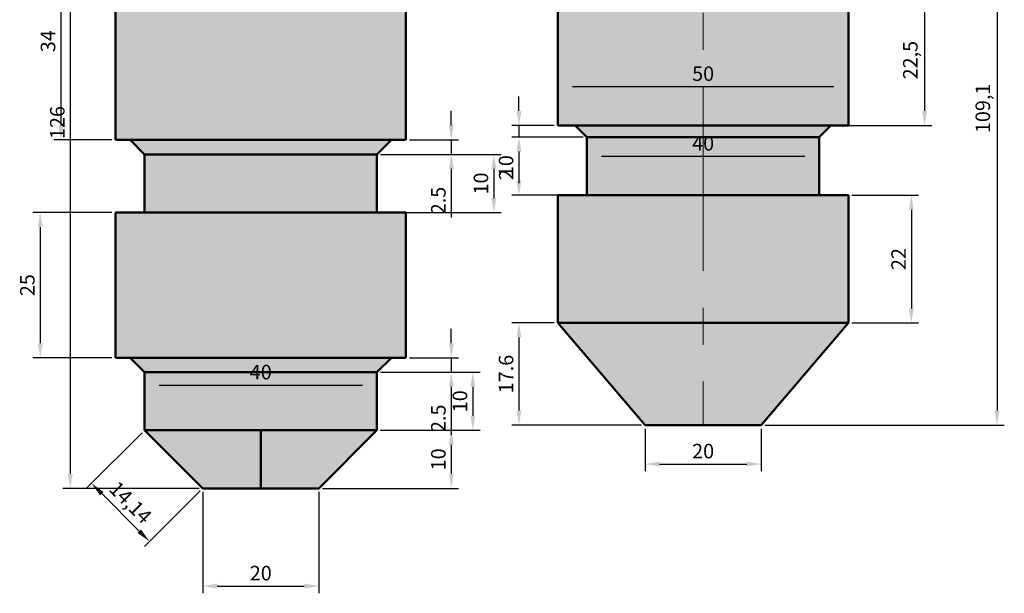
# Model space of a CAD drawing. Units: millimetres. Extents: x 1159 to 1466, y 1237 to 1440.
# Tile 1 of 6: x 1159 to 1329, y 1242 to 1341. Entities that reach past the tile are written whole.
import ezdxf

# ---------------------------------------------------------------- set-up
doc = ezdxf.new("R2010")
doc.units = ezdxf.units.MM
doc.linetypes.add('CENTER', pattern=[50.8, 31.75, -6.35, 6.35, -6.35])
for name, color, linetype, lineweight in [('M-CNTR', 1, 'CENTER', 18), ('M-DIMS', 2, 'Continuous', 25), ('M-HATC', 8, 'Continuous', 18), ('M-OUTL', 7, 'Continuous', 50)]:
    doc.layers.add(name, color=color, linetype=linetype, lineweight=lineweight)
doc.styles.get("Standard").update_dxf_attribs({"font": 'arial.ttf'})
doc.dimstyles.new('ISO-25', dxfattribs={"dimtxt": 2.5, "dimasz": 2.5, "dimexe": 1.25, "dimexo": 0.625, "dimtad": 1, "dimtxsty": 'Standard', "dimcen": 2.5, "dimadec": 0, "dimazin": 0, "dimtfac": 1, "dimtmove": 0, "dimatfit": 3, "dimfxl": 1, "dimarcsym": 0})

# ---------------------------------------------------------------- blocks, each defined once
blk = doc.blocks.new('*D10')
at = {"layer": 'Defpoints', "color": 0, "transparency": 16777216}
for p in [(1190.51, 1260.27), (1210.51, 1260.27), (1210.51, 1243.45)]:
    blk.add_point(p, dxfattribs=at)
at = {"layer": 'M-DIMS', "color": 0, "lineweight": -2, "transparency": 16777216}
for p, q in [((1190.51, 1259.65), (1190.51, 1242.2)), ((1210.51, 1259.65), (1210.51, 1242.2)), ((1193.01, 1243.45), (1208.01, 1243.45))]:
    blk.add_line(p, q, dxfattribs=at)
at = {"layer": 'M-DIMS', "color": 0, "transparency": 16777216}
for points in [[(1193.01, 1243.87), (1193.01, 1243.03), (1190.51, 1243.45)], [(1208.01, 1243.87), (1208.01, 1243.03), (1210.51, 1243.45)]]:
    blk.add_solid(points, dxfattribs=at)
at = {"layer": 'M-DIMS', "color": 0, "transparency": 16777216, "insert": (1200.51, 1245.35), "char_height": 2.5, "attachment_point": 5}
blk.add_mtext('20', dxfattribs=at)
blk = doc.blocks.new('*D12')
at = {"layer": 'Defpoints', "color": 0, "transparency": 16777216}
for p in [(1175.51, 1354.27), (1166.11, 1320.27), (1175.51, 1320.27)]:
    blk.add_point(p, dxfattribs=at)
at = {"layer": 'M-DIMS', "color": 0, "lineweight": -2, "transparency": 16777216}
for p, q in [((1174.88, 1354.27), (1164.86, 1354.27)), ((1166.11, 1351.77), (1166.11, 1322.77)), ((1174.88, 1320.27), (1164.86, 1320.27))]:
    blk.add_line(p, q, dxfattribs=at)
at = {"layer": 'M-DIMS', "color": 0, "transparency": 16777216}
for points in [[(1165.7, 1351.77), (1166.53, 1351.77), (1166.11, 1354.27)], [(1165.7, 1322.77), (1166.53, 1322.77), (1166.11, 1320.27)]]:
    blk.add_solid(points, dxfattribs=at)
at = {"layer": 'M-DIMS', "color": 0, "transparency": 16777216, "insert": (1164.21, 1337.27), "char_height": 2.5, "attachment_point": 5, "rotation": 90}
blk.add_mtext('34', dxfattribs=at)
blk = doc.blocks.new('*D13')
at = {"layer": 'Defpoints', "color": 0, "transparency": 16777216}
for p in [(1220.51, 1317.77), (1220.51, 1307.77), (1240.64, 1307.77)]:
    blk.add_point(p, dxfattribs=at)
at = {"layer": 'M-DIMS', "color": 0, "lineweight": -2, "transparency": 16777216}
for p, q in [((1221.13, 1317.77), (1241.89, 1317.77)), ((1240.64, 1315.27), (1240.64, 1310.27)), ((1221.13, 1307.77), (1241.89, 1307.77))]:
    blk.add_line(p, q, dxfattribs=at)
at = {"layer": 'M-DIMS', "color": 0, "transparency": 16777216}
for points in [[(1240.23, 1315.27), (1241.06, 1315.27), (1240.64, 1317.77)], [(1240.23, 1310.27), (1241.06, 1310.27), (1240.64, 1307.77)]]:
    blk.add_solid(points, dxfattribs=at)
at = {"layer": 'M-DIMS', "color": 0, "transparency": 16777216, "insert": (1238.74, 1312.77), "char_height": 2.5, "attachment_point": 5, "rotation": 90}
blk.add_mtext('10', dxfattribs=at)
blk = doc.blocks.new('*D14')
at = {"layer": 'Defpoints', "color": 0, "transparency": 16777216}
for p in [(1220.51, 1280.27), (1220.51, 1270.27), (1237.02, 1270.27)]:
    blk.add_point(p, dxfattribs=at)
at = {"layer": 'M-DIMS', "color": 0, "lineweight": -2, "transparency": 16777216}
for p, q in [((1221.13, 1280.27), (1238.27, 1280.27)), ((1237.02, 1277.77), (1237.02, 1272.77)), ((1221.13, 1270.27), (1238.27, 1270.27))]:
    blk.add_line(p, q, dxfattribs=at)
at = {"layer": 'M-DIMS', "color": 0, "transparency": 16777216}
for points in [[(1236.6, 1277.77), (1237.43, 1277.77), (1237.02, 1280.27)], [(1236.6, 1272.77), (1237.43, 1272.77), (1237.02, 1270.27)]]:
    blk.add_solid(points, dxfattribs=at)
at = {"layer": 'M-DIMS', "color": 0, "transparency": 16777216, "insert": (1235.12, 1275.27), "char_height": 2.5, "attachment_point": 5, "rotation": 90}
blk.add_mtext('10', dxfattribs=at)
blk = doc.blocks.new('*D15')
at = {"layer": 'Defpoints', "color": 0, "transparency": 16777216}
for p in [(1180.51, 1270.27), (1190.51, 1260.27), (1181.37, 1251.13)]:
    blk.add_point(p, dxfattribs=at)
at = {"layer": 'M-DIMS', "color": 0, "lineweight": -2, "transparency": 16777216}
for p, q in [((1180.07, 1269.83), (1170.48, 1260.24)), ((1190.07, 1259.83), (1180.48, 1250.24)), ((1173.14, 1259.36), (1179.6, 1252.9))]:
    blk.add_line(p, q, dxfattribs=at)
at = {"layer": 'M-DIMS', "color": 0, "transparency": 16777216}
for points in [[(1173.43, 1259.65), (1172.84, 1259.07), (1171.37, 1261.13)], [(1179.89, 1253.19), (1179.31, 1252.6), (1181.37, 1251.13)]]:
    blk.add_solid(points, dxfattribs=at)
at = {"layer": 'M-DIMS', "color": 0, "transparency": 16777216, "insert": (1177.87, 1257.63), "char_height": 2.5, "attachment_point": 5, "rotation": 315}
blk.add_mtext('14,14', dxfattribs=at)
blk = doc.blocks.new('*D16')
at = {"layer": 'Defpoints', "color": 0, "transparency": 16777216}
for p in [(1175.51, 1307.77), (1162.55, 1282.77), (1175.51, 1282.77)]:
    blk.add_point(p, dxfattribs=at)
at = {"layer": 'M-DIMS', "color": 0, "lineweight": -2, "transparency": 16777216}
for p, q in [((1174.88, 1307.77), (1161.3, 1307.77)), ((1162.55, 1305.27), (1162.55, 1285.27)), ((1174.88, 1282.77), (1161.3, 1282.77))]:
    blk.add_line(p, q, dxfattribs=at)
at = {"layer": 'M-DIMS', "color": 0, "transparency": 16777216}
for points in [[(1162.14, 1305.27), (1162.97, 1305.27), (1162.55, 1307.77)], [(1162.14, 1285.27), (1162.97, 1285.27), (1162.55, 1282.77)]]:
    blk.add_solid(points, dxfattribs=at)
at = {"layer": 'M-DIMS', "color": 0, "transparency": 16777216, "insert": (1160.65, 1295.27), "char_height": 2.5, "attachment_point": 5, "rotation": 90}
blk.add_mtext('25', dxfattribs=at)
blk = doc.blocks.new('*D17')
at = {"layer": 'Defpoints', "color": 0, "transparency": 16777216}
for p in [(1291.66, 1380.26), (1286.66, 1271.16), (1327.26, 1271.16)]:
    blk.add_point(p, dxfattribs=at)
at = {"layer": 'M-DIMS', "color": 0, "lineweight": -2, "transparency": 16777216}
for p, q in [((1292.29, 1380.26), (1328.51, 1380.26)), ((1327.26, 1377.76), (1327.26, 1273.66)), ((1287.29, 1271.16), (1328.51, 1271.16))]:
    blk.add_line(p, q, dxfattribs=at)
at = {"layer": 'M-DIMS', "color": 0, "transparency": 16777216}
for points in [[(1326.84, 1377.76), (1327.68, 1377.76), (1327.26, 1380.26)], [(1326.84, 1273.66), (1327.68, 1273.66), (1327.26, 1271.16)]]:
    blk.add_solid(points, dxfattribs=at)
at = {"layer": 'M-DIMS', "color": 0, "transparency": 16777216, "insert": (1325.13, 1325.71), "char_height": 2.5, "attachment_point": 5, "rotation": 90}
blk.add_mtext('109,1', dxfattribs=at)
blk = doc.blocks.new('*D18')
at = {"layer": 'Defpoints', "color": 0, "transparency": 16777216}
for p in [(1301.66, 1345.26), (1300.16, 1322.76), (1314.79, 1322.76)]:
    blk.add_point(p, dxfattribs=at)
at = {"layer": 'M-DIMS', "color": 0, "lineweight": -2, "transparency": 16777216}
for p, q in [((1302.29, 1345.26), (1316.04, 1345.26)), ((1314.79, 1342.76), (1314.79, 1325.26)), ((1300.79, 1322.76), (1316.04, 1322.76))]:
    blk.add_line(p, q, dxfattribs=at)
at = {"layer": 'M-DIMS', "color": 0, "transparency": 16777216}
for points in [[(1314.37, 1342.76), (1315.21, 1342.76), (1314.79, 1345.26)], [(1314.37, 1325.26), (1315.21, 1325.26), (1314.79, 1322.76)]]:
    blk.add_solid(points, dxfattribs=at)
at = {"layer": 'M-DIMS', "color": 0, "transparency": 16777216, "insert": (1312.66, 1334.01), "char_height": 2.5, "attachment_point": 5, "rotation": 90}
blk.add_mtext('22,5', dxfattribs=at)
blk = doc.blocks.new('*D19')
at = {"layer": 'Defpoints', "color": 0, "transparency": 16777216}
for p in [(1301.66, 1310.76), (1301.66, 1288.76), (1312.51, 1288.76)]:
    blk.add_point(p, dxfattribs=at)
at = {"layer": 'M-DIMS', "color": 0, "lineweight": -2, "transparency": 16777216}
for p, q in [((1302.29, 1310.76), (1313.76, 1310.76)), ((1312.51, 1308.26), (1312.51, 1291.26)), ((1302.29, 1288.76), (1313.76, 1288.76))]:
    blk.add_line(p, q, dxfattribs=at)
at = {"layer": 'M-DIMS', "color": 0, "transparency": 16777216}
for points in [[(1312.09, 1308.26), (1312.92, 1308.26), (1312.51, 1310.76)], [(1312.09, 1291.26), (1312.92, 1291.26), (1312.51, 1288.76)]]:
    blk.add_solid(points, dxfattribs=at)
at = {"layer": 'M-DIMS', "color": 0, "transparency": 16777216, "insert": (1310.63, 1299.76), "char_height": 2.5, "attachment_point": 5, "rotation": 90}
blk.add_mtext('22', dxfattribs=at)
blk = doc.blocks.new('*D23')
at = {"layer": 'Defpoints', "color": 0, "transparency": 16777216}
for p in [(1185.51, 1386.27), (1167.71, 1260.27), (1190.51, 1260.27)]:
    blk.add_point(p, dxfattribs=at)
at = {"layer": 'M-DIMS', "color": 0, "lineweight": -2, "transparency": 16777216}
for p, q in [((1184.88, 1386.27), (1166.46, 1386.27)), ((1167.71, 1383.77), (1167.71, 1262.77)), ((1189.88, 1260.27), (1166.46, 1260.27))]:
    blk.add_line(p, q, dxfattribs=at)
at = {"layer": 'M-DIMS', "color": 0, "transparency": 16777216}
for points in [[(1167.29, 1383.77), (1168.13, 1383.77), (1167.71, 1386.27)], [(1167.29, 1262.77), (1168.13, 1262.77), (1167.71, 1260.27)]]:
    blk.add_solid(points, dxfattribs=at)
at = {"layer": 'M-DIMS', "color": 0, "transparency": 16777216, "insert": (1165.81, 1323.27), "char_height": 2.5, "attachment_point": 5, "rotation": 90}
blk.add_mtext('126', dxfattribs=at)
blk = doc.blocks.new('*D25')
at = {"layer": 'Defpoints', "color": 0, "transparency": 16777216}
for p in [(1220.51, 1278.07), (1180.51, 1270.27), (1220.51, 1270.27)]:
    blk.add_point(p, dxfattribs=at)
at = {"layer": 'M-DIMS', "color": 0, "lineweight": -2, "transparency": 16777216}
for p, q in [((1180.51, 1270.9), (1180.51, 1279.32)), ((1183.01, 1278.07), (1218.01, 1278.07)), ((1220.51, 1270.9), (1220.51, 1279.32))]:
    blk.add_line(p, q, dxfattribs=at)
at = {"layer": 'M-DIMS', "color": 0, "transparency": 16777216}
for points in [[(1183.01, 1278.49), (1183.01, 1277.65), (1180.51, 1278.07)], [(1218.01, 1278.49), (1218.01, 1277.65), (1220.51, 1278.07)]]:
    blk.add_solid(points, dxfattribs=at)
at = {"layer": 'M-DIMS', "color": 0, "transparency": 16777216, "insert": (1200.51, 1279.97), "char_height": 2.5, "attachment_point": 5}
blk.add_mtext('40', dxfattribs=at)
blk = doc.blocks.new('*D26')
at = {"layer": 'Defpoints', "color": 0, "transparency": 16777216}
for p in [(1225.51, 1320.27), (1220.51, 1317.77), (1233.31, 1317.77)]:
    blk.add_point(p, dxfattribs=at)
at = {"layer": 'M-DIMS', "color": 0, "lineweight": -2, "transparency": 16777216}
for p, q in [((1233.31, 1322.77), (1233.31, 1325.27)), ((1226.13, 1320.27), (1234.56, 1320.27)), ((1233.31, 1320.27), (1233.31, 1317.77)), ((1221.13, 1317.77), (1234.56, 1317.77)), ((1233.31, 1315.27), (1233.31, 1306.91))]:
    blk.add_line(p, q, dxfattribs=at)
at = {"layer": 'M-DIMS', "color": 0, "transparency": 16777216}
for points in [[(1232.89, 1322.77), (1233.73, 1322.77), (1233.31, 1320.27)], [(1232.89, 1315.27), (1233.73, 1315.27), (1233.31, 1317.77)]]:
    blk.add_solid(points, dxfattribs=at)
at = {"layer": 'M-DIMS', "color": 0, "transparency": 16777216, "insert": (1231.41, 1309.84), "char_height": 2.5, "attachment_point": 5, "rotation": 90}
blk.add_mtext('2.5', dxfattribs=at)
blk = doc.blocks.new('*D27')
at = {"layer": 'Defpoints', "color": 0, "transparency": 16777216}
for p in [(1225.51, 1282.77), (1220.51, 1280.27), (1233.31, 1280.27)]:
    blk.add_point(p, dxfattribs=at)
at = {"layer": 'M-DIMS', "color": 0, "lineweight": -2, "transparency": 16777216}
for p, q in [((1233.31, 1285.27), (1233.31, 1287.77)), ((1226.13, 1282.77), (1234.56, 1282.77)), ((1233.31, 1282.77), (1233.31, 1280.27)), ((1221.13, 1280.27), (1234.56, 1280.27)), ((1233.31, 1277.77), (1233.31, 1269.41))]:
    blk.add_line(p, q, dxfattribs=at)
at = {"layer": 'M-DIMS', "color": 0, "transparency": 16777216}
for points in [[(1232.89, 1285.27), (1233.73, 1285.27), (1233.31, 1282.77)], [(1232.89, 1277.77), (1233.73, 1277.77), (1233.31, 1280.27)]]:
    blk.add_solid(points, dxfattribs=at)
at = {"layer": 'M-DIMS', "color": 0, "transparency": 16777216, "insert": (1231.41, 1272.34), "char_height": 2.5, "attachment_point": 5, "rotation": 90}
blk.add_mtext('2.5', dxfattribs=at)
blk = doc.blocks.new('*D28')
at = {"layer": 'Defpoints', "color": 0, "transparency": 16777216}
for p in [(1220.51, 1270.27), (1210.51, 1260.27), (1233.31, 1260.27)]:
    blk.add_point(p, dxfattribs=at)
at = {"layer": 'M-DIMS', "color": 0, "lineweight": -2, "transparency": 16777216}
for p, q in [((1221.13, 1270.27), (1234.56, 1270.27)), ((1233.31, 1267.77), (1233.31, 1262.77)), ((1211.13, 1260.27), (1234.56, 1260.27))]:
    blk.add_line(p, q, dxfattribs=at)
at = {"layer": 'M-DIMS', "color": 0, "transparency": 16777216}
for points in [[(1232.89, 1267.77), (1233.73, 1267.77), (1233.31, 1270.27)], [(1232.89, 1262.77), (1233.73, 1262.77), (1233.31, 1260.27)]]:
    blk.add_solid(points, dxfattribs=at)
at = {"layer": 'M-DIMS', "color": 0, "transparency": 16777216, "insert": (1231.41, 1265.27), "char_height": 2.5, "attachment_point": 5, "rotation": 90}
blk.add_mtext('10', dxfattribs=at)
blk = doc.blocks.new('*D30')
at = {"layer": 'Defpoints', "color": 0, "transparency": 16777216}
for p in [(1301.66, 1329.46), (1251.66, 1322.76), (1301.66, 1322.76)]:
    blk.add_point(p, dxfattribs=at)
at = {"layer": 'M-DIMS', "color": 0, "lineweight": -2, "transparency": 16777216}
for p, q in [((1251.66, 1323.39), (1251.66, 1330.71)), ((1301.66, 1323.39), (1301.66, 1330.71)), ((1254.16, 1329.46), (1299.16, 1329.46))]:
    blk.add_line(p, q, dxfattribs=at)
at = {"layer": 'M-DIMS', "color": 0, "transparency": 16777216}
for points in [[(1254.16, 1329.88), (1254.16, 1329.04), (1251.66, 1329.46)], [(1299.16, 1329.88), (1299.16, 1329.04), (1301.66, 1329.46)]]:
    blk.add_solid(points, dxfattribs=at)
at = {"layer": 'M-DIMS', "color": 0, "transparency": 16777216, "insert": (1276.66, 1331.36), "char_height": 2.5, "attachment_point": 5}
blk.add_mtext('50', dxfattribs=at)
blk = doc.blocks.new('*D31')
at = {"layer": 'Defpoints', "color": 0, "transparency": 16777216}
for p in [(1296.66, 1317.46), (1256.66, 1310.76), (1296.66, 1310.76)]:
    blk.add_point(p, dxfattribs=at)
at = {"layer": 'M-DIMS', "color": 0, "lineweight": -2, "transparency": 16777216}
for p, q in [((1256.66, 1311.39), (1256.66, 1318.71)), ((1259.16, 1317.46), (1294.16, 1317.46)), ((1296.66, 1311.39), (1296.66, 1318.71))]:
    blk.add_line(p, q, dxfattribs=at)
at = {"layer": 'M-DIMS', "color": 0, "transparency": 16777216}
for points in [[(1259.16, 1317.88), (1259.16, 1317.04), (1256.66, 1317.46)], [(1294.16, 1317.88), (1294.16, 1317.04), (1296.66, 1317.46)]]:
    blk.add_solid(points, dxfattribs=at)
at = {"layer": 'M-DIMS', "color": 0, "transparency": 16777216, "insert": (1276.66, 1319.36), "char_height": 2.5, "attachment_point": 5}
blk.add_mtext('40', dxfattribs=at)
blk = doc.blocks.new('*D32')
at = {"layer": 'Defpoints', "color": 0, "transparency": 16777216}
for p in [(1266.66, 1271.16), (1286.66, 1271.16), (1286.66, 1264.46)]:
    blk.add_point(p, dxfattribs=at)
at = {"layer": 'M-DIMS', "color": 0, "lineweight": -2, "transparency": 16777216}
for p, q in [((1266.66, 1270.53), (1266.66, 1263.21)), ((1286.66, 1270.53), (1286.66, 1263.21)), ((1269.16, 1264.46), (1284.16, 1264.46))]:
    blk.add_line(p, q, dxfattribs=at)
at = {"layer": 'M-DIMS', "color": 0, "transparency": 16777216}
for points in [[(1269.16, 1264.88), (1269.16, 1264.04), (1266.66, 1264.46)], [(1284.16, 1264.88), (1284.16, 1264.04), (1286.66, 1264.46)]]:
    blk.add_solid(points, dxfattribs=at)
at = {"layer": 'M-DIMS', "color": 0, "transparency": 16777216, "insert": (1276.66, 1266.36), "char_height": 2.5, "attachment_point": 5}
blk.add_mtext('20', dxfattribs=at)
blk = doc.blocks.new('*D34')
at = {"layer": 'Defpoints', "color": 0, "transparency": 16777216}
for p in [(1256.66, 1320.76), (1244.96, 1310.76), (1256.66, 1310.76)]:
    blk.add_point(p, dxfattribs=at)
at = {"layer": 'M-DIMS', "color": 0, "lineweight": -2, "transparency": 16777216}
for p, q in [((1256.04, 1320.76), (1243.71, 1320.76)), ((1244.96, 1318.26), (1244.96, 1313.26)), ((1256.04, 1310.76), (1243.71, 1310.76))]:
    blk.add_line(p, q, dxfattribs=at)
at = {"layer": 'M-DIMS', "color": 0, "transparency": 16777216}
for points in [[(1244.54, 1318.26), (1245.38, 1318.26), (1244.96, 1320.76)], [(1244.54, 1313.26), (1245.38, 1313.26), (1244.96, 1310.76)]]:
    blk.add_solid(points, dxfattribs=at)
at = {"layer": 'M-DIMS', "color": 0, "transparency": 16777216, "insert": (1243.06, 1315.76), "char_height": 2.5, "attachment_point": 5, "rotation": 90}
blk.add_mtext('10', dxfattribs=at)
blk = doc.blocks.new('*D35')
at = {"layer": 'Defpoints', "color": 0, "transparency": 16777216}
for p in [(1251.66, 1322.76), (1244.96, 1320.76), (1256.66, 1320.76)]:
    blk.add_point(p, dxfattribs=at)
at = {"layer": 'M-DIMS', "color": 0, "lineweight": -2, "transparency": 16777216}
for p, q in [((1244.96, 1325.26), (1244.96, 1327.76)), ((1251.04, 1322.76), (1243.71, 1322.76)), ((1244.96, 1322.76), (1244.96, 1320.76)), ((1256.04, 1320.76), (1243.71, 1320.76)), ((1244.96, 1318.26), (1244.96, 1312.85))]:
    blk.add_line(p, q, dxfattribs=at)
at = {"layer": 'M-DIMS', "color": 0, "transparency": 16777216}
for points in [[(1244.54, 1325.26), (1245.38, 1325.26), (1244.96, 1322.76)], [(1244.54, 1318.26), (1245.38, 1318.26), (1244.96, 1320.76)]]:
    blk.add_solid(points, dxfattribs=at)
at = {"layer": 'M-DIMS', "color": 0, "transparency": 16777216, "insert": (1243.08, 1314.31), "char_height": 2.5, "attachment_point": 5, "rotation": 90}
blk.add_mtext('2', dxfattribs=at)
blk = doc.blocks.new('*D36')
at = {"layer": 'Defpoints', "color": 0, "transparency": 16777216}
for p in [(1251.66, 1288.76), (1244.96, 1271.16), (1266.66, 1271.16)]:
    blk.add_point(p, dxfattribs=at)
at = {"layer": 'M-DIMS', "color": 0, "lineweight": -2, "transparency": 16777216}
for p, q in [((1251.04, 1288.76), (1243.71, 1288.76)), ((1244.96, 1286.26), (1244.96, 1273.66)), ((1266.04, 1271.16), (1243.71, 1271.16))]:
    blk.add_line(p, q, dxfattribs=at)
at = {"layer": 'M-DIMS', "color": 0, "transparency": 16777216}
for points in [[(1244.54, 1286.26), (1245.38, 1286.26), (1244.96, 1288.76)], [(1244.54, 1273.66), (1245.38, 1273.66), (1244.96, 1271.16)]]:
    blk.add_solid(points, dxfattribs=at)
at = {"layer": 'M-DIMS', "color": 0, "transparency": 16777216, "insert": (1243.06, 1279.96), "char_height": 2.5, "attachment_point": 5, "rotation": 90}
blk.add_mtext('17.6', dxfattribs=at)

msp = doc.modelspace()

# ---------------------------------------------------------------- hatches: boundary and pattern name
at = {"layer": 'M-HATC'}
h = msp.add_hatch(color=256, dxfattribs=at)
h.set_gradient(color1=(254, 204, 102), color2=(254, 204, 102))
h.paths.add_polyline_path([(1215.5099, 1386.2704), (1185.5099, 1386.2704), (1185.5099, 1354.2704), (1215.5099, 1354.2704)])
h.paths.add_polyline_path([(1225.5099, 1354.2704), (1215.5099, 1354.2704), (1185.5099, 1354.2704), (1175.5099, 1354.2704), (1175.5099, 1320.2704), (1178.0099, 1320.2704), (1223.0099, 1320.2704), (1225.5099, 1320.2704)])
h.paths.add_polyline_path([(1200.5099, 1270.2704), (1180.5099, 1270.2704), (1190.5099, 1260.2704), (1200.5099, 1260.2704)])
h.paths.add_polyline_path([(1220.5099, 1270.2704), (1200.5099, 1270.2704), (1200.5099, 1260.2704), (1210.5099, 1260.2704)])
h = msp.add_hatch(color=256, dxfattribs=at)
h.set_gradient(color1=(237, 31, 36), color2=(248, 215, 49))
h.paths.add_polyline_path([(1276.6615, 1345.2603), (1261.6615, 1345.2603), (1251.6615, 1345.2603), (1251.6615, 1322.7603), (1254.6615, 1322.7603), (1276.6615, 1322.7603)])
h.paths.add_polyline_path([(1301.6615, 1345.2603), (1291.6615, 1345.2603), (1276.6615, 1345.2603), (1276.6615, 1322.7603), (1298.6615, 1322.7603), (1301.6615, 1322.7603)])
h = msp.add_hatch(color=256, dxfattribs=at)
h.set_gradient(color1=(0, 0, 255), color2=(0, 0, 255))
h.paths.add_polyline_path([(1276.6615, 1322.7603), (1254.6615, 1322.7603), (1256.6615, 1320.7603), (1276.6615, 1320.7603)])
h.paths.add_polyline_path([(1298.6615, 1322.7603), (1276.6615, 1322.7603), (1276.6615, 1320.7603), (1296.6615, 1320.7603)])
h = msp.add_hatch(color=256, dxfattribs=at)
h.set_gradient(color1=(153, 155, 55), color2=(153, 155, 55))
h.paths.add_polyline_path([(1276.6615, 1320.7603), (1256.6615, 1320.7603), (1256.6615, 1310.7603), (1276.6615, 1310.7603)])
h.paths.add_polyline_path([(1296.6615, 1320.7603), (1276.6615, 1320.7603), (1276.6615, 1310.7603), (1296.6615, 1310.7603)])
h = msp.add_hatch(color=256, dxfattribs=at)
h.set_gradient(color1=(248, 153, 30), color2=(248, 153, 30))
h.paths.add_polyline_path([(1178.0099, 1320.2704), (1180.5099, 1317.7704), (1220.5099, 1317.7704), (1223.0099, 1320.2704)])
h = msp.add_hatch(color=256, dxfattribs=at)
h.set_gradient(color1=(99, 100, 102), color2=(99, 100, 102))
h.paths.add_polyline_path([(1220.5099, 1307.7704), (1220.5099, 1317.7704), (1180.5099, 1317.7704), (1180.5099, 1307.7704)])
h = msp.add_hatch(color=256, dxfattribs=at)
h.set_gradient(color1=(205, 105, 40), color2=(153, 155, 55))
h.paths.add_polyline_path([(1276.6615, 1310.7603), (1256.6615, 1310.7603), (1251.6615, 1310.7603), (1251.6615, 1288.7603), (1276.6615, 1288.7603)])
h.paths.add_polyline_path([(1301.6615, 1310.7603), (1296.6615, 1310.7603), (1276.6615, 1310.7603), (1276.6615, 1288.7603), (1291.6615, 1288.7603), (1296.6615, 1288.7603), (1301.6615, 1288.7603)])
h = msp.add_hatch(color=256, dxfattribs=at)
h.set_gradient(color1=(100, 33, 101), color2=(100, 33, 101))
h.paths.add_polyline_path([(1180.5099, 1307.7704), (1175.5099, 1307.7704), (1175.5099, 1282.7704), (1178.0099, 1282.7704), (1223.0099, 1282.7704), (1225.5099, 1282.7704), (1225.5099, 1307.7704), (1220.5099, 1307.7704)])
h = msp.add_hatch(color=256, dxfattribs=at)
h.set_gradient(color1=(34, 52, 110), color2=(0, 0, 0))
h.paths.add_polyline_path([(1276.6615, 1288.7603), (1251.6615, 1288.7603), (1266.6615, 1271.159), (1276.6615, 1271.159)])
h.paths.add_polyline_path([(1301.6615, 1288.7603), (1296.6615, 1288.7603), (1291.6615, 1288.7603), (1276.6615, 1288.7603), (1276.6615, 1271.159), (1286.6615, 1271.159)])
h = msp.add_hatch(color=256, dxfattribs=at)
h.set_gradient(color1=(255, 255, 255))
h.paths.add_polyline_path([(1220.5099, 1280.2704), (1223.0099, 1282.7704), (1178.0099, 1282.7704), (1180.5099, 1280.2704)])
h = msp.add_hatch(color=256, dxfattribs=at)
h.set_gradient(color1=(19, 103, 52), color2=(19, 103, 52))
h.paths.add_polyline_path([(1180.5099, 1280.2704), (1180.5099, 1270.2704), (1220.5099, 1270.2704), (1220.5099, 1280.2704)])

# ---------------------------------------------------------------- linework, layer by layer
at = {"layer": 'M-CNTR'}
msp.add_line((1276.6615, 1380.2603), (1276.6615, 1271.159), dxfattribs=at)
at = {"layer": 'M-OUTL'}
for p, q in [((1175.5099, 1354.2704), (1175.5099, 1320.2704)), ((1225.5099, 1320.2704), (1225.5099, 1354.2704)), ((1251.6615, 1345.2603), (1251.6615, 1322.7603)), ((1301.6615, 1322.7603), (1301.6615, 1345.2603)), ((1251.6615, 1322.7603), (1254.6615, 1322.7603)), ((1256.6615, 1320.7603), (1254.6615, 1322.7603)), ((1254.6615, 1322.7603), (1298.6615, 1322.7603)), ((1296.6615, 1320.7603), (1298.6615, 1322.7603)), ((1298.6615, 1322.7603), (1301.6615, 1322.7603)), ((1256.6615, 1320.7603), (1256.6615, 1320.7603)), ((1256.6615, 1320.7603), (1296.6615, 1320.7603)), ((1256.6615, 1320.7603), (1256.6615, 1310.7603)), ((1296.6615, 1320.7603), (1296.6615, 1320.7603)), ((1296.6615, 1310.7603), (1296.6615, 1320.7603)), ((1175.5099, 1320.2704), (1178.0099, 1320.2704)), ((1180.5099, 1317.7704), (1178.0099, 1320.2704)), ((1178.0099, 1320.2704), (1223.0099, 1320.2704)), ((1220.5099, 1317.7704), (1223.0099, 1320.2704)), ((1223.0099, 1320.2704), (1225.5099, 1320.2704)), ((1180.5099, 1317.7704), (1180.5099, 1317.7704)), ((1180.5099, 1317.7704), (1220.5099, 1317.7704)), ((1180.5099, 1317.7704), (1180.5099, 1307.7704)), ((1220.5099, 1317.7704), (1220.5099, 1317.7704)), ((1220.5099, 1307.7704), (1220.5099, 1317.7704)), ((1256.6615, 1310.7603), (1251.6615, 1310.7603)), ((1251.6615, 1310.7603), (1251.6615, 1288.7603)), ((1256.6615, 1310.7603), (1296.6615, 1310.7603)), ((1301.6615, 1310.7603), (1296.6615, 1310.7603)), ((1301.6615, 1288.7603), (1301.6615, 1310.7603)), ((1180.5099, 1307.7704), (1175.5099, 1307.7704)), ((1175.5099, 1307.7704), (1175.5099, 1282.7704)), ((1180.5099, 1307.7704), (1220.5099, 1307.7704)), ((1225.5099, 1307.7704), (1220.5099, 1307.7704)), ((1225.5099, 1282.7704), (1225.5099, 1307.7704)), ((1251.6615, 1288.7603), (1291.6615, 1288.7603)), ((1266.6615, 1271.159), (1251.6615, 1288.7603)), ((1286.6615, 1271.159), (1301.6615, 1288.7603)), ((1291.6615, 1288.7603), (1296.6615, 1288.7603)), ((1296.6615, 1288.7603), (1301.6615, 1288.7603)), ((1175.5099, 1282.7704), (1178.0099, 1282.7704)), ((1180.5099, 1280.2704), (1178.0099, 1282.7704)), ((1178.0099, 1282.7704), (1223.0099, 1282.7704)), ((1220.5099, 1280.2704), (1223.0099, 1282.7704)), ((1223.0099, 1282.7704), (1225.5099, 1282.7704)), ((1180.5099, 1280.2704), (1180.5099, 1280.2704)), ((1180.5099, 1280.2704), (1220.5099, 1280.2704)), ((1180.5099, 1280.2704), (1180.5099, 1270.2704)), ((1220.5099, 1280.2704), (1220.5099, 1280.2704)), ((1220.5099, 1270.2704), (1220.5099, 1280.2704)), ((1180.5099, 1270.2704), (1220.5099, 1270.2704)), ((1180.5099, 1270.2704), (1190.5099, 1260.2704)), ((1200.5099, 1270.2704), (1200.5099, 1260.2704)), ((1220.5099, 1270.2704), (1210.5099, 1260.2704)), ((1276.6615, 1271.159), (1266.6615, 1271.159)), ((1276.6615, 1271.159), (1286.6615, 1271.159)), ((1200.5099, 1260.2704), (1190.5099, 1260.2704)), ((1200.5099, 1260.2704), (1210.5099, 1260.2704))]:
    msp.add_line(p, q, dxfattribs=at)

# ---------------------------------------------------------------- dimensions: what is measured, and where the dimension line sits
at = {"layer": 'M-DIMS'}
for base, p1, p2, override, picture, middle in [((1167.7099, 1260.2704), (1185.5099, 1386.2704), (1190.5099, 1260.2704), {"dimdec": 0, "dimlfac": 1, "dimrnd": 0, "dimzin": 0, "dimdsep": 46, "dimlunit": 2}, '*D23', (1165.8085, 1323.2704)), ((1327.2609, 1271.159), (1291.6615, 1380.2603), (1286.6615, 1271.159), {"dimclrd": 0, "dimclre": 0, "dimclrt": 0}, '*D17', (1325.1335, 1325.7096)), ((1166.1136, 1320.2704), (1175.5099, 1354.2704), (1175.5099, 1320.2704), {"dimclrd": 0, "dimclre": 0, "dimclrt": 0}, '*D12', (1164.2113, 1337.2704)), ((1314.79, 1322.7603), (1301.6615, 1345.2603), (1300.1615, 1322.7603), {"dimclrd": 0, "dimclre": 0, "dimclrt": 0}, '*D18', (1312.6626, 1334.0103)), ((1244.9615, 1320.7603), (1251.6615, 1322.7603), (1256.6615, 1320.7603), {"dimdec": 0, "dimlfac": 1, "dimrnd": 0, "dimzin": 0, "dimdsep": 46, "dimlunit": 2}, '*D35', (1243.0814, 1314.3073)), ((1233.3099, 1317.7704), (1225.5099, 1320.2704), (1220.5099, 1317.7704), {"dimdec": 1, "dimlfac": 1, "dimrnd": 0, "dimzin": 0, "dimdsep": 46, "dimlunit": 2}, '*D26', (1231.4085, 1309.8389)), ((1244.9615, 1310.7603), (1256.6615, 1320.7603), (1256.6615, 1310.7603), {"dimdec": 0, "dimlfac": 1, "dimrnd": 0, "dimzin": 0, "dimdsep": 46, "dimlunit": 2}, '*D34', (1243.0601, 1315.7603)), ((1240.6419, 1307.7704), (1220.5099, 1317.7704), (1220.5099, 1307.7704), {"dimclrd": 0, "dimclre": 0, "dimclrt": 0}, '*D13', (1238.7405, 1312.7704)), ((1312.5066, 1288.7603), (1301.6615, 1310.7603), (1301.6615, 1288.7603), {"dimclrd": 0, "dimclre": 0, "dimclrt": 0}, '*D19', (1310.6265, 1299.7603)), ((1162.5527, 1282.7704), (1175.5099, 1307.7704), (1175.5099, 1282.7704), {"dimclrd": 0, "dimclre": 0, "dimclrt": 0}, '*D16', (1160.6512, 1295.2704)), ((1244.9615, 1271.159), (1251.6615, 1288.7603), (1266.6615, 1271.159), {"dimdec": 1, "dimlfac": 1, "dimrnd": 0, "dimzin": 0, "dimdsep": 46, "dimlunit": 2}, '*D36', (1243.0601, 1279.9596)), ((1233.3099, 1280.2704), (1225.5099, 1282.7704), (1220.5099, 1280.2704), {"dimdec": 1, "dimlfac": 1, "dimrnd": 0, "dimzin": 0, "dimdsep": 46, "dimlunit": 2}, '*D27', (1231.4085, 1272.3389)), ((1237.0174, 1270.2704), (1220.5099, 1280.2704), (1220.5099, 1270.2704), {"dimclrd": 0, "dimclre": 0, "dimclrt": 0}, '*D14', (1235.116, 1275.2704)), ((1233.3099, 1260.2704), (1220.5099, 1270.2704), (1210.5099, 1260.2704), {"dimdec": 0, "dimlfac": 1, "dimrnd": 0, "dimzin": 0, "dimdsep": 46, "dimlunit": 2}, '*D28', (1231.4085, 1265.2704))]:
    dim = msp.add_linear_dim(base=base, p1=p1, p2=p2, angle=90, dimstyle='ISO-25', override=override, dxfattribs=at)
    dim.commit()
    dim.dimension.update_dxf_attribs({"geometry": picture, "text_midpoint": middle})
for base, p1, p2, override, picture, middle in [((1301.6615, 1329.4603), (1251.6615, 1322.7603), (1301.6615, 1322.7603), {"dimdec": 0, "dimlfac": 1, "dimrnd": 0, "dimzin": 0, "dimdsep": 46, "dimlunit": 2}, '*D30', (1276.6615, 1331.3617)), ((1296.6615, 1317.4603), (1256.6615, 1310.7603), (1296.6615, 1310.7603), {"dimdec": 0, "dimlfac": 1, "dimrnd": 0, "dimzin": 0, "dimdsep": 46, "dimlunit": 2}, '*D31', (1276.6615, 1319.3617)), ((1220.5099, 1278.0704), (1180.5099, 1270.2704), (1220.5099, 1270.2704), {"dimdec": 0, "dimlfac": 1, "dimrnd": 0, "dimzin": 0, "dimdsep": 46, "dimlunit": 2}, '*D25', (1200.5099, 1279.9718)), ((1286.6615, 1264.459), (1266.6615, 1271.159), (1286.6615, 1271.159), {"dimdec": 0, "dimlfac": 1, "dimrnd": 0, "dimzin": 0, "dimdsep": 46, "dimlunit": 2}, '*D32', (1276.6615, 1266.3604)), ((1210.5099, 1243.4496), (1190.5099, 1260.2704), (1210.5099, 1260.2704), {"dimclrd": 0, "dimclre": 0, "dimclrt": 0}, '*D10', (1200.5099, 1245.351))]:
    dim = msp.add_linear_dim(base=base, p1=p1, p2=p2, dimstyle='ISO-25', override=override, dxfattribs=at)
    dim.commit()
    dim.dimension.update_dxf_attribs({"geometry": picture, "text_midpoint": middle})
dim = msp.add_aligned_dim(p1=(1180.5099, 1270.2704), p2=(1190.5099, 1260.2704), distance=-12.9294, dimstyle='ISO-25', override={"dimclrd": 0, "dimclre": 0, "dimclrt": 0}, dxfattribs=at)
dim.commit()
dim.dimension.update_dxf_attribs({"geometry": '*D15', "text_midpoint": (1177.8718, 1257.6322)})

doc.saveas('drawing.dxf')
